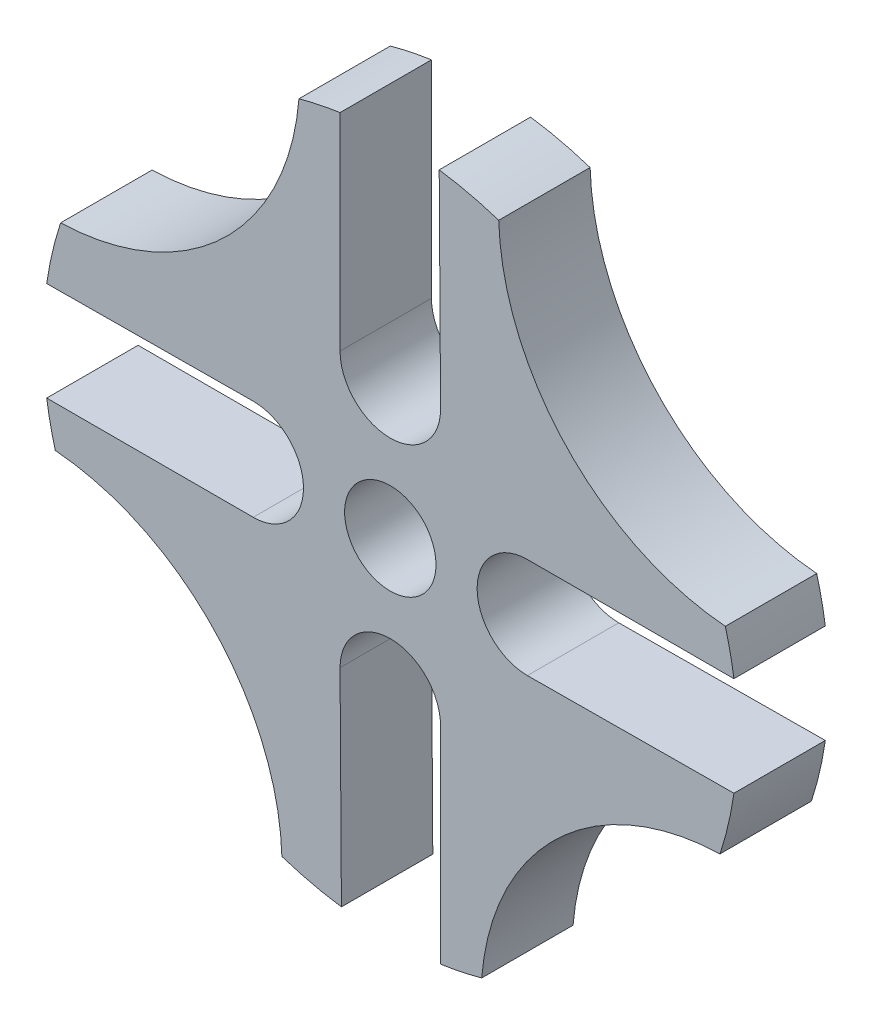
from build123d import *

# Parameters (mm, degrees)
GENEVA_WHEEL_PROFILE_R       = 5
GENEVA_WHEEL_BODY_10MM_DEPTH = 10


with BuildPart() as part:
    # Geneva Wheel Profile → Geneva Wheel Body 10mm (new body)
    with BuildSketch(Plane.XY):
        with BuildLine():
            ThreePointArc((-36.078505425, 11.862749321), (-18.305680685, 19.283646977), (-10, 36.66060556))
            ThreePointArc((-10, 36.66060556), (-7.764216189, 37.198346025), (-5.5, 37.599867021))
            Line((-5.5, 37.599867021), (-5.5, 15))
            ThreePointArc((-5.5, 15), (0, 9.5), (5.5, 15))
            Line((5.5, 15), (5.350081788, 37.6))
            ThreePointArc((5.350081788, 37.6), (8.639972519, 36.982891315), (11.862749321, 36.078505425))
            ThreePointArc((11.862749321, 36.078505425), (19.283646977, 18.305680685), (36.66060556, 10))
            ThreePointArc((36.66060556, 10), (37.198346025, 7.764216189), (37.599867021, 5.5))
            Line((37.599867021, 5.5), (15, 5.5))
            ThreePointArc((15, 5.5), (9.5, 0), (15, -5.5))
            Line((15, -5.5), (37.6, -5.350081788))
            ThreePointArc((37.6, -5.350081788), (36.982891315, -8.639972519), (36.078505425, -11.862749321))
            ThreePointArc((36.078505425, -11.862749321), (18.305680685, -19.283646977), (10, -36.66060556))
            ThreePointArc((10, -36.66060556), (7.764216189, -37.198346025), (5.5, -37.599867021))
            Line((5.5, -37.599867021), (5.5, -15))
            ThreePointArc((5.5, -15), (0, -9.5), (-5.5, -15))
            Line((-5.5, -15), (-5.350081788, -37.6))
            ThreePointArc((-5.350081788, -37.6), (-8.639972519, -36.982891315), (-11.862749321, -36.078505425))
            ThreePointArc((-11.862749321, -36.078505425), (-19.283646977, -18.305680685), (-36.66060556, -10))
            ThreePointArc((-36.66060556, -10), (-37.198346025, -7.764216189), (-37.599867021, -5.5))
            Line((-37.599867021, -5.5), (-15, -5.5))
            ThreePointArc((-15, -5.5), (-9.5, 0), (-15, 5.5))
            Line((-15, 5.5), (-37.6, 5.350081788))
            ThreePointArc((-37.6, 5.350081788), (-36.982891315, 8.639972519), (-36.078505425, 11.862749321))
        make_face()
        Circle(GENEVA_WHEEL_PROFILE_R, mode=Mode.SUBTRACT)
    extrude(amount=GENEVA_WHEEL_BODY_10MM_DEPTH)


solid = part.part
